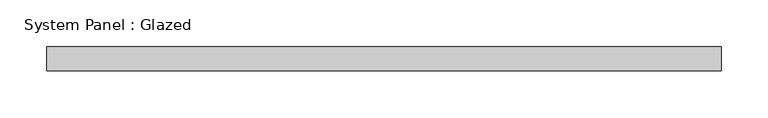
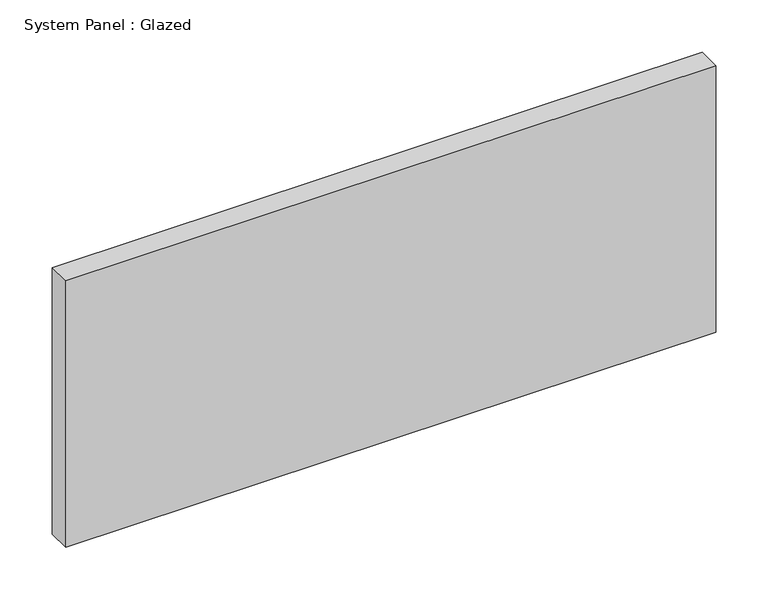
"""IFC4 building model written with IfcOpenShell, lengths in millimetres: plate geometry, System Panel : Glazed."""

from ifc_helpers import new_model, si_unit, origin, origin_with_axes, place, context, project, spatial, polyline, outline, extrude, source, transform, mapped, element, save


def system_panel_glazed_fef3bb39(model_context):
    return source(origin(), model_context, "Body", "SweptSolid", [
        extrude(outline(polyline([(358.775, 19.05), (-358.775, 19.05), (-358.775, 44.45), (358.775, 44.45), (358.775, 19.05)])), origin_with_axes(), (0.0, 0.0, 1.0), 311.15),
    ])


if __name__ == "__main__":
    model = new_model("IFC4")
    model_context = context("Model", 3, world=origin())
    ifc_project = project(units=[si_unit("LENGTHUNIT", "METRE", prefix="MILLI")], contexts=[model_context])
    site = spatial("IfcSite", under=ifc_project)
    building = spatial("IfcBuilding", under=site)
    placement = place(None, origin())
    system_panel_glazed_shape = system_panel_glazed_fef3bb39(model_context)
    element("IfcPlate", 1, ObjectType="System Panel : Glazed", at=placement, inside=building, context=model_context, shape_type="MappedRepresentation", body=[
        mapped(system_panel_glazed_shape, transform((0.0, 0.0, 0.0), x_axis=(1.0, 0.0, 0.0), y_axis=(0.0, 1.0, 0.0), z_axis=(0.0, 0.0, 1.0))),
    ])
    save(model, "model.ifc")

# Revit data of these elements
# Type "System Panel : Glazed"
#   Construction Type Id = "GSP4R"
#   Analytic Construction = "1/8 in Pilkington single glazing"
#   Visual Light Transmittance = 0.9
#   Solar Heat Gain Coefficient = 0.86
#   Heat Transfer Coefficient (U) = 1.18115 BTU/(h·ft²·°F)
#   Define Thermal Properties by = 1
# Element 1 (IfcPlate, "System Panel : Glazed")
#   Materials on its faces: "Glass"
# Materials
#   "Glass": class "Glass", colour RGB 0 128 192, transparency 0.75, Description = "Soda Lime Glass", Cost = 0
